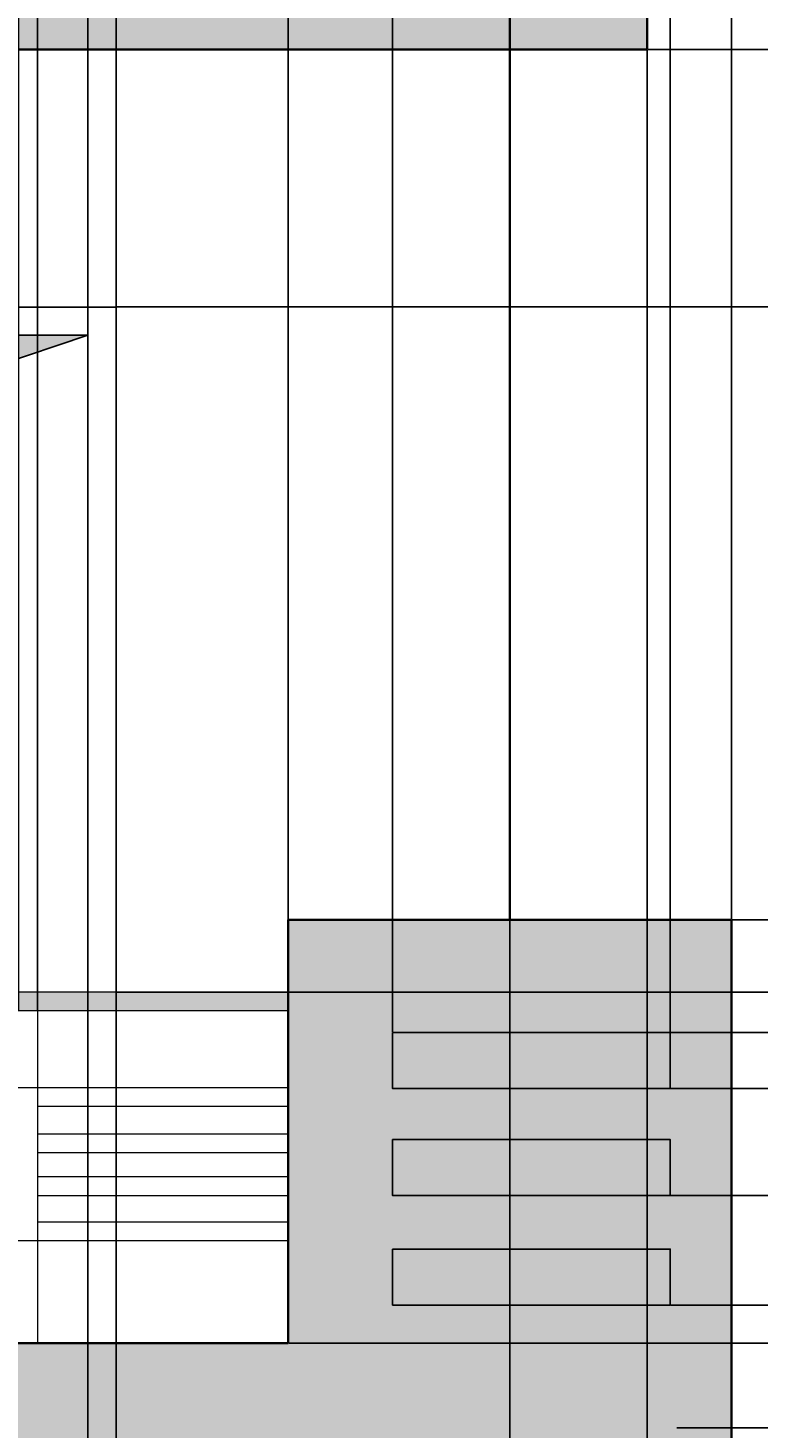
# Model space of a CAD drawing. Units: inches. Extents: x 62 to 566, y 66 to 528.
# Tile 17 of 20: x 365 to 443, y 298 to 447. Entities that reach past the tile are written whole.
import ezdxf

# ---------------------------------------------------------------- set-up
doc = ezdxf.new("R2010")
doc.units = ezdxf.units.IN
doc.header["$MEASUREMENT"] = 0
for name, color, linetype, lineweight in [('A-ANNO-DIMS', 2, 'Continuous', 18), ('A-DOOR', 4, 'Continuous', 25), ('A-ELEV', 7, 'Continuous', 35), ('A-FLOR-HRAL', 6, 'Continuous', 18), ('A-GLAZ', 3, 'Continuous', 25), ('A-WALL-PATT', 8, 'Continuous', 13)]:
    doc.layers.add(name, color=color, linetype=linetype, lineweight=lineweight)
doc.styles.get("Standard").update_dxf_attribs({"font": 'arial.ttf'})
doc.dimstyles.get("Standard").update_dxf_attribs({"dimtxt": 0.75, "dimasz": 0.18, "dimexe": 0.18, "dimexo": 0.0625, "dimgap": 0.09, "dimtad": 0, "dimtih": 1, "dimtoh": 1, "dimdec": 4, "dimzin": 0, "dimdsep": 46, "dimlunit": 4, "dimtxsty": 'Standard', "dimcen": 0.09, "dimadec": 0, "dimazin": 0, "dimtfac": 1, "dimtdec": 4, "dimtofl": 0, "dimtmove": 0, "dimatfit": 3, "dimfxl": 1, "dimtolj": 1, "dimtzin": 0, "dimarcsym": 0})

# ---------------------------------------------------------------- blocks, each defined once
blk = doc.blocks.new('*D23')
at = {"layer": 'A-ANNO-DIMS', "color": 0, "lineweight": -2, "transparency": 16777216}
for p, q in [((374.2, 344.78), (564.47, 344.78)), ((564.29, 344.6), (564.29, 308.57)), ((564.29, 271.59), (564.29, 307.62)), ((540.1, 271.41), (564.47, 271.41))]:
    blk.add_line(p, q, dxfattribs=at)
at = {"layer": 'A-ANNO-DIMS', "color": 0, "transparency": 16777216}
for points in [[(564.26, 344.6), (564.32, 344.6), (564.29, 344.78)], [(564.26, 271.59), (564.32, 271.59), (564.29, 271.41)]]:
    blk.add_solid(points, dxfattribs=at)
at = {"layer": 'Defpoints', "color": 0, "transparency": 16777216}
for p in [(374.14, 344.78), (564.29, 344.78), (540.04, 271.41)]:
    blk.add_point(p, dxfattribs=at)
at = {"layer": 'A-ANNO-DIMS', "color": 0, "transparency": 16777216, "insert": (564.29, 308.1), "char_height": 0.75, "attachment_point": 5}
blk.add_mtext('\\A1;73.37', dxfattribs=at)
blk = doc.blocks.new('*D24')
at = {"layer": 'A-ANNO-DIMS', "color": 0, "lineweight": -2, "transparency": 16777216}
for p, q in [((374.2, 417.71), (564.47, 417.71)), ((564.29, 417.53), (564.29, 381.72)), ((564.29, 344.96), (564.29, 380.77)), ((374.2, 344.78), (564.47, 344.78))]:
    blk.add_line(p, q, dxfattribs=at)
at = {"layer": 'A-ANNO-DIMS', "color": 0, "transparency": 16777216}
for points in [[(564.26, 417.53), (564.32, 417.53), (564.29, 417.71)], [(564.26, 344.96), (564.32, 344.96), (564.29, 344.78)]]:
    blk.add_solid(points, dxfattribs=at)
at = {"layer": 'Defpoints', "color": 0, "transparency": 16777216}
for p in [(374.14, 417.71), (564.29, 417.71), (374.14, 344.78)]:
    blk.add_point(p, dxfattribs=at)
at = {"layer": 'A-ANNO-DIMS', "color": 0, "transparency": 16777216, "insert": (564.29, 381.24), "char_height": 0.75, "attachment_point": 5}
blk.add_mtext('\\A1;72.92', dxfattribs=at)
blk = doc.blocks.new('*D41')
at = {"layer": 'A-ANNO-DIMS', "color": 0, "lineweight": -2, "transparency": 16777216}
for p, q in [((316.21, 417.64), (316.21, 65.94)), ((374.14, 417.64), (374.14, 65.94)), ((316.39, 66.12), (343.82, 66.12)), ((373.96, 66.12), (346.53, 66.12))]:
    blk.add_line(p, q, dxfattribs=at)
at = {"layer": 'A-ANNO-DIMS', "color": 0, "transparency": 16777216}
for points in [[(316.39, 66.15), (316.39, 66.09), (316.21, 66.12)], [(373.96, 66.15), (373.96, 66.09), (374.14, 66.12)]]:
    blk.add_solid(points, dxfattribs=at)
at = {"layer": 'Defpoints', "color": 0, "transparency": 16777216}
for p in [(316.21, 417.71), (374.14, 417.71), (374.14, 66.12)]:
    blk.add_point(p, dxfattribs=at)
at = {"layer": 'A-ANNO-DIMS', "color": 0, "transparency": 16777216, "insert": (345.17, 66.12), "char_height": 0.75, "attachment_point": 5}
blk.add_mtext('\\A1;57.93', dxfattribs=at)
blk = doc.blocks.new('*D42')
at = {"layer": 'A-ANNO-DIMS', "color": 0, "lineweight": -2, "transparency": 16777216}
for p, q in [((416.08, 445.04), (416.08, 65.94)), ((374.14, 417.64), (374.14, 65.94)), ((374.32, 66.12), (393.74, 66.12)), ((415.9, 66.12), (396.48, 66.12))]:
    blk.add_line(p, q, dxfattribs=at)
at = {"layer": 'A-ANNO-DIMS', "color": 0, "transparency": 16777216}
for points in [[(374.32, 66.15), (374.32, 66.09), (374.14, 66.12)], [(415.9, 66.15), (415.9, 66.09), (416.08, 66.12)]]:
    blk.add_solid(points, dxfattribs=at)
at = {"layer": 'Defpoints', "color": 0, "transparency": 16777216}
for p in [(416.08, 445.11), (374.14, 417.71), (416.08, 66.12)]:
    blk.add_point(p, dxfattribs=at)
at = {"layer": 'A-ANNO-DIMS', "color": 0, "transparency": 16777216, "insert": (395.11, 66.12), "char_height": 0.75, "attachment_point": 5}
blk.add_mtext('\\A1;41.95', dxfattribs=at)
blk = doc.blocks.new('*D43')
at = {"layer": 'A-ANNO-DIMS', "color": 0, "lineweight": -2, "transparency": 16777216}
for p, q in [((416.08, 445.04), (416.08, 65.94)), ((430.69, 445.04), (430.69, 65.94)), ((416.26, 66.12), (422.14, 66.12)), ((430.51, 66.12), (424.64, 66.12))]:
    blk.add_line(p, q, dxfattribs=at)
at = {"layer": 'A-ANNO-DIMS', "color": 0, "transparency": 16777216}
for points in [[(416.26, 66.15), (416.26, 66.09), (416.08, 66.12)], [(430.51, 66.15), (430.51, 66.09), (430.69, 66.12)]]:
    blk.add_solid(points, dxfattribs=at)
at = {"layer": 'Defpoints', "color": 0, "transparency": 16777216}
for p in [(416.08, 445.11), (430.69, 445.11), (430.69, 66.12)]:
    blk.add_point(p, dxfattribs=at)
at = {"layer": 'A-ANNO-DIMS', "color": 0, "transparency": 16777216, "insert": (423.39, 66.12), "char_height": 0.75, "attachment_point": 5}
blk.add_mtext('\\A1;14.61', dxfattribs=at)
blk = doc.blocks.new('*D52')
at = {"layer": 'A-ANNO-DIMS', "color": 0, "lineweight": -2, "transparency": 16777216}
for p, q in [((430.76, 445.11), (564.47, 445.11)), ((564.29, 444.93), (564.29, 431.87)), ((564.29, 417.89), (564.29, 430.94)), ((374.2, 417.71), (564.47, 417.71))]:
    blk.add_line(p, q, dxfattribs=at)
at = {"layer": 'A-ANNO-DIMS', "color": 0, "transparency": 16777216}
for points in [[(564.26, 444.93), (564.32, 444.93), (564.29, 445.11)], [(564.26, 417.89), (564.32, 417.89), (564.29, 417.71)]]:
    blk.add_solid(points, dxfattribs=at)
at = {"layer": 'Defpoints', "color": 0, "transparency": 16777216}
for p in [(430.69, 445.11), (564.29, 445.11), (374.14, 417.71)]:
    blk.add_point(p, dxfattribs=at)
at = {"layer": 'A-ANNO-DIMS', "color": 0, "transparency": 16777216, "insert": (564.29, 431.41), "char_height": 0.75, "attachment_point": 5}
blk.add_mtext('\\A1;27.4', dxfattribs=at)
blk = doc.blocks.new('*D53')
at = {"layer": 'A-ANNO-DIMS', "color": 0, "lineweight": -2, "transparency": 16777216}
for p, q in [((430.76, 462.04), (564.47, 462.04)), ((564.29, 461.86), (564.29, 454.05)), ((564.29, 445.29), (564.29, 453.1)), ((430.76, 445.11), (564.47, 445.11))]:
    blk.add_line(p, q, dxfattribs=at)
at = {"layer": 'A-ANNO-DIMS', "color": 0, "transparency": 16777216}
for points in [[(564.26, 461.86), (564.32, 461.86), (564.29, 462.04)], [(564.26, 445.29), (564.32, 445.29), (564.29, 445.11)]]:
    blk.add_solid(points, dxfattribs=at)
at = {"layer": 'Defpoints', "color": 0, "transparency": 16777216}
for p in [(430.69, 462.04), (564.29, 462.04), (430.69, 445.11)]:
    blk.add_point(p, dxfattribs=at)
at = {"layer": 'A-ANNO-DIMS', "color": 0, "transparency": 16777216, "insert": (564.29, 453.57), "char_height": 0.75, "attachment_point": 5}
blk.add_mtext('\\A1;16.936', dxfattribs=at)
blk = doc.blocks.new('*D63')
at = {"layer": 'A-ANNO-DIMS', "color": 0, "lineweight": -2, "transparency": 16777216}
for p, q in [((329.67, 219.79), (329.67, 527.47)), ((371.14, 233.72), (371.14, 527.47)), ((329.85, 527.29), (349.03, 527.29)), ((370.96, 527.29), (351.77, 527.29))]:
    blk.add_line(p, q, dxfattribs=at)
at = {"layer": 'A-ANNO-DIMS', "color": 0, "transparency": 16777216}
for points in [[(329.85, 527.32), (329.85, 527.26), (329.67, 527.29)], [(370.96, 527.32), (370.96, 527.26), (371.14, 527.29)]]:
    blk.add_solid(points, dxfattribs=at)
at = {"layer": 'Defpoints', "color": 0, "transparency": 16777216}
for p in [(371.14, 527.29), (371.14, 233.66), (329.67, 219.73)]:
    blk.add_point(p, dxfattribs=at)
at = {"layer": 'A-ANNO-DIMS', "color": 0, "transparency": 16777216, "insert": (350.4, 527.29), "char_height": 0.75, "attachment_point": 5}
blk.add_mtext('\\A1;41.47', dxfattribs=at)
blk = doc.blocks.new('*D64')
at = {"layer": 'A-ANNO-DIMS', "color": 0, "lineweight": -2, "transparency": 16777216}
for p, q in [((371.14, 233.72), (371.14, 527.47)), ((374.14, 236.72), (374.14, 527.47)), ((371.32, 527.29), (372.3, 527.29)), ((373.96, 527.29), (372.97, 527.29))]:
    blk.add_line(p, q, dxfattribs=at)
at = {"layer": 'A-ANNO-DIMS', "color": 0, "transparency": 16777216}
for points in [[(371.32, 527.32), (371.32, 527.26), (371.14, 527.29)], [(373.96, 527.32), (373.96, 527.26), (374.14, 527.29)]]:
    blk.add_solid(points, dxfattribs=at)
at = {"layer": 'Defpoints', "color": 0, "transparency": 16777216}
for p in [(374.14, 527.29), (374.14, 236.66), (371.14, 233.66)]:
    blk.add_point(p, dxfattribs=at)
at = {"layer": 'A-ANNO-DIMS', "color": 0, "transparency": 16777216, "insert": (372.64, 527.29), "char_height": 0.75, "attachment_point": 5}
blk.add_mtext('\\A1;3', dxfattribs=at)
blk = doc.blocks.new('*D77')
at = {"layer": 'A-ANNO-DIMS', "color": 0, "lineweight": -2, "transparency": 16777216}
for p, q in [((363.76, 342.84), (363.76, 527.47)), ((365.76, 342.84), (365.76, 527.47)), ((363.94, 527.29), (364.43, 527.29)), ((365.58, 527.29), (365.1, 527.29))]:
    blk.add_line(p, q, dxfattribs=at)
at = {"layer": 'A-ANNO-DIMS', "color": 0, "transparency": 16777216}
for points in [[(363.94, 527.32), (363.94, 527.26), (363.76, 527.29)], [(365.58, 527.32), (365.58, 527.26), (365.76, 527.29)]]:
    blk.add_solid(points, dxfattribs=at)
at = {"layer": 'Defpoints', "color": 0, "transparency": 16777216}
for p in [(365.76, 527.29), (363.76, 342.78), (365.76, 342.78)]:
    blk.add_point(p, dxfattribs=at)
at = {"layer": 'A-ANNO-DIMS', "color": 0, "transparency": 16777216, "insert": (364.76, 527.29), "char_height": 0.75, "attachment_point": 5}
blk.add_mtext('\\A1;2', dxfattribs=at)
blk = doc.blocks.new('*D78')
at = {"layer": 'A-ANNO-DIMS', "color": 0, "lineweight": -2, "transparency": 16777216}
for p, q in [((365.76, 342.84), (365.76, 527.47)), ((392.48, 342.84), (392.48, 527.47)), ((365.94, 527.29), (377.47, 527.29)), ((392.3, 527.29), (380.78, 527.29))]:
    blk.add_line(p, q, dxfattribs=at)
at = {"layer": 'A-ANNO-DIMS', "color": 0, "transparency": 16777216}
for points in [[(365.94, 527.32), (365.94, 527.26), (365.76, 527.29)], [(392.3, 527.32), (392.3, 527.26), (392.48, 527.29)]]:
    blk.add_solid(points, dxfattribs=at)
at = {"layer": 'Defpoints', "color": 0, "transparency": 16777216}
for p in [(392.48, 527.29), (365.76, 342.78), (392.48, 342.78)]:
    blk.add_point(p, dxfattribs=at)
at = {"layer": 'A-ANNO-DIMS', "color": 0, "transparency": 16777216, "insert": (379.12, 527.29), "char_height": 0.75, "attachment_point": 5}
blk.add_mtext('\\A1;26.715', dxfattribs=at)
blk = doc.blocks.new('*D79')
at = {"layer": 'A-ANNO-DIMS', "color": 0, "lineweight": -2, "transparency": 16777216}
for p, q in [((392.48, 352.55), (392.48, 527.47)), ((403.58, 340.55), (403.58, 527.47)), ((392.66, 527.29), (396.42, 527.29)), ((403.4, 527.29), (399.64, 527.29))]:
    blk.add_line(p, q, dxfattribs=at)
at = {"layer": 'A-ANNO-DIMS', "color": 0, "transparency": 16777216}
for points in [[(392.66, 527.32), (392.66, 527.26), (392.48, 527.29)], [(403.4, 527.32), (403.4, 527.26), (403.58, 527.29)]]:
    blk.add_solid(points, dxfattribs=at)
at = {"layer": 'Defpoints', "color": 0, "transparency": 16777216}
for p in [(403.58, 527.29), (392.48, 352.48), (403.58, 340.49)]:
    blk.add_point(p, dxfattribs=at)
at = {"layer": 'A-ANNO-DIMS', "color": 0, "transparency": 16777216, "insert": (398.03, 527.29), "char_height": 0.75, "attachment_point": 5}
blk.add_mtext('\\A1;11.106', dxfattribs=at)
blk = doc.blocks.new('*D80')
at = {"layer": 'A-ANNO-DIMS', "color": 0, "lineweight": -2, "transparency": 16777216}
for p, q in [((403.58, 340.55), (403.58, 527.47)), ((433.16, 340.55), (433.16, 527.47)), ((403.76, 527.29), (417.01, 527.29)), ((432.98, 527.29), (419.74, 527.29))]:
    blk.add_line(p, q, dxfattribs=at)
at = {"layer": 'A-ANNO-DIMS', "color": 0, "transparency": 16777216}
for points in [[(403.76, 527.32), (403.76, 527.26), (403.58, 527.29)], [(432.98, 527.32), (432.98, 527.26), (433.16, 527.29)]]:
    blk.add_solid(points, dxfattribs=at)
at = {"layer": 'Defpoints', "color": 0, "transparency": 16777216}
for p in [(433.16, 527.29), (403.58, 340.49), (433.16, 340.49)]:
    blk.add_point(p, dxfattribs=at)
at = {"layer": 'A-ANNO-DIMS', "color": 0, "transparency": 16777216, "insert": (418.37, 527.29), "char_height": 0.75, "attachment_point": 5}
blk.add_mtext('\\A1;29.58', dxfattribs=at)
blk = doc.blocks.new('*D81')
at = {"layer": 'A-ANNO-DIMS', "color": 0, "lineweight": -2, "transparency": 16777216}
for p, q in [((433.16, 340.55), (433.16, 527.47)), ((439.69, 352.55), (439.69, 527.47)), ((433.34, 527.29), (435.07, 527.29)), ((439.51, 527.29), (437.78, 527.29))]:
    blk.add_line(p, q, dxfattribs=at)
at = {"layer": 'A-ANNO-DIMS', "color": 0, "transparency": 16777216}
for points in [[(433.34, 527.32), (433.34, 527.26), (433.16, 527.29)], [(439.51, 527.32), (439.51, 527.26), (439.69, 527.29)]]:
    blk.add_solid(points, dxfattribs=at)
at = {"layer": 'Defpoints', "color": 0, "transparency": 16777216}
for p in [(439.69, 527.29), (439.69, 352.48), (433.16, 340.49)]:
    blk.add_point(p, dxfattribs=at)
at = {"layer": 'A-ANNO-DIMS', "color": 0, "transparency": 16777216, "insert": (436.43, 527.29), "char_height": 0.75, "attachment_point": 5}
blk.add_mtext('\\A1;6.524', dxfattribs=at)
blk = doc.blocks.new('*D91')
at = {"layer": 'A-ANNO-DIMS', "color": 0, "lineweight": -2, "transparency": 16777216}
for p, q in [((433.87, 298.4), (564.47, 298.4)), ((564.29, 298.22), (564.29, 297.15)), ((564.29, 295.13), (564.29, 296.2)), ((433.87, 294.95), (564.47, 294.95))]:
    blk.add_line(p, q, dxfattribs=at)
at = {"layer": 'A-ANNO-DIMS', "color": 0, "transparency": 16777216}
for points in [[(564.26, 298.22), (564.32, 298.22), (564.29, 298.4)], [(564.26, 295.13), (564.32, 295.13), (564.29, 294.95)]]:
    blk.add_solid(points, dxfattribs=at)
at = {"layer": 'Defpoints', "color": 0, "transparency": 16777216}
for p in [(433.81, 298.4), (564.29, 298.4), (433.81, 294.95)]:
    blk.add_point(p, dxfattribs=at)
at = {"layer": 'A-ANNO-DIMS', "color": 0, "transparency": 16777216, "insert": (564.29, 296.67), "char_height": 0.75, "attachment_point": 5}
blk.add_mtext('\\A1;3.449', dxfattribs=at)
blk = doc.blocks.new('*D92')
at = {"layer": 'A-ANNO-DIMS', "color": 0, "lineweight": -2, "transparency": 16777216}
for p, q in [((392.54, 307.41), (564.47, 307.41)), ((564.29, 307.23), (564.29, 303.38)), ((564.29, 298.58), (564.29, 302.43)), ((433.87, 298.4), (564.47, 298.4))]:
    blk.add_line(p, q, dxfattribs=at)
at = {"layer": 'A-ANNO-DIMS', "color": 0, "transparency": 16777216}
for points in [[(564.26, 307.23), (564.32, 307.23), (564.29, 307.41)], [(564.26, 298.58), (564.32, 298.58), (564.29, 298.4)]]:
    blk.add_solid(points, dxfattribs=at)
at = {"layer": 'Defpoints', "color": 0, "transparency": 16777216}
for p in [(392.48, 307.41), (564.29, 307.41), (433.81, 298.4)]:
    blk.add_point(p, dxfattribs=at)
at = {"layer": 'A-ANNO-DIMS', "color": 0, "transparency": 16777216, "insert": (564.29, 302.91), "char_height": 0.75, "attachment_point": 5}
blk.add_mtext('\\A1;9.014', dxfattribs=at)
blk = doc.blocks.new('*D93')
at = {"layer": 'A-ANNO-DIMS', "color": 0, "lineweight": -2, "transparency": 16777216}
for p, q in [((433.23, 311.47), (564.47, 311.47)), ((564.29, 311.29), (564.29, 309.92)), ((564.29, 307.59), (564.29, 308.97)), ((392.54, 307.41), (564.47, 307.41))]:
    blk.add_line(p, q, dxfattribs=at)
at = {"layer": 'A-ANNO-DIMS', "color": 0, "transparency": 16777216}
for points in [[(564.26, 311.29), (564.32, 311.29), (564.29, 311.47)], [(564.26, 307.59), (564.32, 307.59), (564.29, 307.41)]]:
    blk.add_solid(points, dxfattribs=at)
at = {"layer": 'Defpoints', "color": 0, "transparency": 16777216}
for p in [(433.16, 311.47), (564.29, 311.47), (392.48, 307.41)]:
    blk.add_point(p, dxfattribs=at)
at = {"layer": 'A-ANNO-DIMS', "color": 0, "transparency": 16777216, "insert": (564.29, 309.44), "char_height": 0.75, "attachment_point": 5}
blk.add_mtext('\\A1;4.061', dxfattribs=at)
blk = doc.blocks.new('*D94')
at = {"layer": 'A-ANNO-DIMS', "color": 0, "lineweight": -2, "transparency": 16777216}
for p, q in [((433.23, 323.13), (564.47, 323.13)), ((564.29, 322.95), (564.29, 317.78)), ((564.29, 311.65), (564.29, 316.83)), ((433.23, 311.47), (564.47, 311.47))]:
    blk.add_line(p, q, dxfattribs=at)
at = {"layer": 'A-ANNO-DIMS', "color": 0, "transparency": 16777216}
for points in [[(564.26, 322.95), (564.32, 322.95), (564.29, 323.13)], [(564.26, 311.65), (564.32, 311.65), (564.29, 311.47)]]:
    blk.add_solid(points, dxfattribs=at)
at = {"layer": 'Defpoints', "color": 0, "transparency": 16777216}
for p in [(433.16, 323.13), (564.29, 323.13), (433.16, 311.47)]:
    blk.add_point(p, dxfattribs=at)
at = {"layer": 'A-ANNO-DIMS', "color": 0, "transparency": 16777216, "insert": (564.29, 317.3), "char_height": 0.75, "attachment_point": 5}
blk.add_mtext('\\A1;11.66', dxfattribs=at)
blk = doc.blocks.new('*D95')
at = {"layer": 'A-ANNO-DIMS', "color": 0, "lineweight": -2, "transparency": 16777216}
for p, q in [((433.23, 334.52), (564.47, 334.52)), ((564.29, 334.34), (564.29, 329.3)), ((564.29, 323.31), (564.29, 328.35)), ((433.23, 323.13), (564.47, 323.13))]:
    blk.add_line(p, q, dxfattribs=at)
at = {"layer": 'A-ANNO-DIMS', "color": 0, "transparency": 16777216}
for points in [[(564.26, 334.34), (564.32, 334.34), (564.29, 334.52)], [(564.26, 323.31), (564.32, 323.31), (564.29, 323.13)]]:
    blk.add_solid(points, dxfattribs=at)
at = {"layer": 'Defpoints', "color": 0, "transparency": 16777216}
for p in [(433.16, 334.52), (564.29, 334.52), (433.16, 323.13)]:
    blk.add_point(p, dxfattribs=at)
at = {"layer": 'A-ANNO-DIMS', "color": 0, "transparency": 16777216, "insert": (564.29, 328.83), "char_height": 0.75, "attachment_point": 5}
blk.add_mtext('\\A1;11.388', dxfattribs=at)
blk = doc.blocks.new('*D96')
at = {"layer": 'A-ANNO-DIMS', "color": 0, "lineweight": -2, "transparency": 16777216}
for p, q in [((433.23, 340.49), (564.47, 340.49)), ((564.29, 340.31), (564.29, 337.98)), ((564.29, 334.7), (564.29, 337.03)), ((433.23, 334.52), (564.47, 334.52))]:
    blk.add_line(p, q, dxfattribs=at)
at = {"layer": 'A-ANNO-DIMS', "color": 0, "transparency": 16777216}
for points in [[(564.26, 340.31), (564.32, 340.31), (564.29, 340.49)], [(564.26, 334.7), (564.32, 334.7), (564.29, 334.52)]]:
    blk.add_solid(points, dxfattribs=at)
at = {"layer": 'Defpoints', "color": 0, "transparency": 16777216}
for p in [(433.16, 340.49), (564.29, 340.49), (433.16, 334.52)]:
    blk.add_point(p, dxfattribs=at)
at = {"layer": 'A-ANNO-DIMS', "color": 0, "transparency": 16777216, "insert": (564.29, 337.5), "char_height": 0.75, "attachment_point": 5}
blk.add_mtext('\\A1;5.965', dxfattribs=at)
blk = doc.blocks.new('*D97')
at = {"layer": 'A-ANNO-DIMS', "color": 0, "lineweight": -2, "transparency": 16777216}
for p, q in [((439.75, 352.48), (564.47, 352.48)), ((564.29, 352.3), (564.29, 346.96)), ((564.29, 340.67), (564.29, 346.01)), ((433.23, 340.49), (564.47, 340.49))]:
    blk.add_line(p, q, dxfattribs=at)
at = {"layer": 'A-ANNO-DIMS', "color": 0, "transparency": 16777216}
for points in [[(564.26, 352.3), (564.32, 352.3), (564.29, 352.48)], [(564.26, 340.67), (564.32, 340.67), (564.29, 340.49)]]:
    blk.add_solid(points, dxfattribs=at)
at = {"layer": 'Defpoints', "color": 0, "transparency": 16777216}
for p in [(439.69, 352.48), (564.29, 352.48), (433.16, 340.49)]:
    blk.add_point(p, dxfattribs=at)
at = {"layer": 'A-ANNO-DIMS', "color": 0, "transparency": 16777216, "insert": (564.29, 346.49), "char_height": 0.75, "attachment_point": 5}
blk.add_mtext('\\A1;11.998', dxfattribs=at)

msp = doc.modelspace()

# ---------------------------------------------------------------- hatches: boundary and pattern name
at = {"layer": 'A-WALL-PATT'}
h = msp.add_hatch(color=256, dxfattribs=at)
h.dxf.hatch_style = 1
h.paths.add_polyline_path([(416.0836, 462.0423), (125.9418, 462.0423), (125.9418, 414.3686), (125.9418, 270.3686), (125.9418, 126.3686), (142.3851, 126.3686), (142.3851, 270.3686), (142.3851, 414.3686), (142.3851, 445.1064), (284.2021, 445.1064), (416.0836, 445.1064)])
h.paths.add_polyline_path([(435.3945, 503.0423), (426.3652, 503.0423), (120.4058, 503.0423), (120.4058, 501.0423), (125.9418, 501.0423), (416.0836, 501.0423), (426.3652, 501.0423), (430.6938, 501.0423), (435.3945, 501.0423)])
h.paths.add_polyline_path([(439.6878, 352.4848), (392.4793, 352.4848), (392.4793, 307.4128), (217.2752, 307.4128), (217.2752, 295.4098), (217.2752, 271.4128), (272.0586, 271.4128), (439.6878, 271.4128)])
h.paths.add_polyline_path([(248.0143, 297.1682), (255.6783, 297.1682), (255.6783, 280.0423), (248.0143, 280.0423)], flags=16)
h.paths.add_polyline_path([(235.4641, 280.0423), (227.8001, 280.0423), (227.8001, 297.1682), (235.4641, 297.1682)], flags=16)
h.paths.add_polyline_path([(270.4427, 297.1682), (278.1067, 297.1682), (278.1067, 280.0423), (270.4427, 280.0423)], flags=16)
h.paths.add_polyline_path([(296.3755, 297.1682), (304.0395, 297.1682), (304.0395, 280.0423), (296.3755, 280.0423)], flags=16)
h.paths.add_polyline_path([(319.2543, 297.1682), (326.9183, 297.1682), (326.9183, 280.0423), (319.2543, 280.0423)], flags=16)
h.paths.add_polyline_path([(341.2622, 297.1682), (348.9262, 297.1682), (348.9262, 280.0423), (341.2622, 280.0423)], flags=16)
h.paths.add_polyline_path([(389.2857, 298.3985), (433.8102, 298.3985), (433.8102, 294.9497), (389.2857, 294.9497)], flags=16)
h.paths.add_polyline_path([(389.2857, 291.6038), (433.8102, 291.6038), (433.8102, 288.155), (389.2857, 288.155)], flags=16)
h.paths.add_polyline_path([(389.2857, 284.9607), (433.8102, 284.9607), (433.8102, 281.5119), (389.2857, 281.5119)], flags=16)
h.paths.add_polyline_path([(403.5849, 311.4736), (403.5849, 317.4388), (433.1636, 317.4388), (433.1636, 311.4736)], flags=16)
h.paths.add_polyline_path([(403.5849, 323.1329), (403.5849, 329.0982), (433.1636, 329.0982), (433.1636, 323.1329)], flags=16)
h.paths.add_polyline_path([(403.5849, 334.5211), (403.5849, 340.4863), (433.1636, 340.4863), (433.1636, 334.5211)], flags=16)
h.paths.add_polyline_path([(272.0586, 160.3545), (217.2752, 160.3545), (217.2752, 129.0504), (217.2752, 126.3686), (272.0586, 126.3686)], flags=17)
h.paths.add_polyline_path([(220.5897, 149.5749), (220.5897, 152.296), (267.7931, 152.296), (267.7931, 149.5749)], flags=16)
h.paths.add_polyline_path([(267.7931, 146.6724), (267.7931, 143.9513), (220.5897, 143.9513), (220.5897, 146.6724)], flags=16)
h.paths.add_polyline_path([(220.5897, 155.3799), (220.5897, 158.101), (267.7931, 158.101), (267.7931, 155.3799)], flags=16)
h.paths.add_polyline_path([(267.7931, 140.686), (267.7931, 137.9649), (220.5897, 137.9649), (220.5897, 140.686)], flags=16)
h.paths.add_polyline_path([(267.7931, 135.516), (267.7931, 132.7949), (220.5897, 132.7949), (220.5897, 135.516)], flags=16)
h = msp.add_hatch(color=256, dxfattribs=at)
h.dxf.hatch_style = 1
h.paths.add_polyline_path([(416.0836, 501.0423), (282.3509, 501.0423), (282.3509, 465.0423), (416.0836, 465.0423)])
h.paths.add_polyline_path([(284.2021, 420.597), (272.0586, 420.597), (272.0586, 309.5388), (272.0586, 307.4128), (284.2021, 307.4128)], flags=17)
h.paths.add_polyline_path([(284.2021, 445.1064), (142.3851, 445.1064), (142.3851, 414.3686), (142.3851, 270.3686), (142.3851, 126.3686), (163.6548, 126.3686), (163.6548, 270.5016), (163.6548, 414.5016), (163.6548, 427.4752), (284.2021, 427.4752)])
h.paths.add_polyline_path([(235.4641, 297.1682), (227.8001, 297.1682), (227.8001, 280.0423), (235.4641, 280.0423)], flags=17)
h.paths.add_polyline_path([(255.6783, 297.1682), (248.0143, 297.1682), (248.0143, 280.0423), (255.6783, 280.0423)], flags=17)
h.paths.add_polyline_path([(278.1067, 297.1682), (270.4427, 297.1682), (270.4427, 280.0423), (278.1067, 280.0423)], flags=17)
h.paths.add_polyline_path([(304.0395, 297.1682), (296.3755, 297.1682), (296.3755, 280.0423), (304.0395, 280.0423)])
h.paths.add_polyline_path([(326.9183, 297.1682), (319.2543, 297.1682), (319.2543, 280.0423), (326.9183, 280.0423)])
h.paths.add_polyline_path([(348.9262, 297.1682), (341.2622, 297.1682), (341.2622, 280.0423), (348.9262, 280.0423)])
h.paths.add_polyline_path([(433.8102, 284.9607), (389.2857, 284.9607), (389.2857, 281.5119), (433.8102, 281.5119)])
h.paths.add_polyline_path([(433.8102, 291.6038), (389.2857, 291.6038), (389.2857, 288.155), (433.8102, 288.155)])
h.paths.add_polyline_path([(433.8102, 298.3985), (389.2857, 298.3985), (389.2857, 294.9497), (433.8102, 294.9497)])
h.paths.add_polyline_path([(433.1636, 317.4388), (403.5849, 317.4388), (403.5849, 311.4736), (433.1636, 311.4736)])
h.paths.add_polyline_path([(433.1636, 329.0982), (403.5849, 329.0982), (403.5849, 323.1329), (433.1636, 323.1329)])
h.paths.add_polyline_path([(433.1636, 340.4863), (403.5849, 340.4863), (403.5849, 334.5211), (433.1636, 334.5211)])
h.paths.add_polyline_path([(284.2021, 271.4128), (272.0586, 271.4128), (272.0586, 160.3545), (272.0586, 126.3686), (284.2021, 126.3686)])
h.paths.add_polyline_path([(267.7931, 158.101), (220.5897, 158.101), (220.5897, 155.3799), (267.7931, 155.3799)], flags=17)
h.paths.add_polyline_path([(267.7931, 152.296), (220.5897, 152.296), (220.5897, 149.5749), (267.7931, 149.5749)], flags=17)
h.paths.add_polyline_path([(267.7931, 146.6724), (220.5897, 146.6724), (220.5897, 143.9513), (267.7931, 143.9513)], flags=17)
h.paths.add_polyline_path([(267.7931, 140.686), (220.5897, 140.686), (220.5897, 137.9649), (267.7931, 137.9649)], flags=17)
h.paths.add_polyline_path([(267.7931, 135.516), (220.5897, 135.516), (220.5897, 132.7949), (267.7931, 132.7949)], flags=17)
h.paths.add_polyline_path([(148.2354, 493.4274), (140.5713, 493.4274), (140.5713, 476.3015), (148.2354, 476.3015)])
h.paths.add_polyline_path([(163.2545, 493.4274), (155.5905, 493.4274), (155.5905, 476.3015), (163.2545, 476.3015)])
h.paths.add_polyline_path([(177.9243, 493.7764), (170.2603, 493.7764), (170.2603, 476.6506), (177.9243, 476.6506)])
h.paths.add_polyline_path([(193.9913, 493.7764), (186.3273, 493.7764), (186.3273, 476.6506), (193.9913, 476.6506)])
h.paths.add_polyline_path([(209.709, 493.7764), (202.045, 493.7764), (202.045, 476.6506), (209.709, 476.6506)])
h = msp.add_hatch(color=256, dxfattribs=at)
h.dxf.hatch_style = 1
h.paths.add_polyline_path([(430.6938, 462.0423), (416.0836, 462.0423), (416.0836, 445.1064), (430.6938, 445.1064)])
h.paths.add_polyline_path([(169.0431, 420.597), (284.2021, 420.597), (284.2021, 426.4752), (164.6548, 426.4752), (164.6548, 414.5016), (164.6548, 126.3686), (169.0431, 126.3686)])
h = msp.add_hatch(color=256, dxfattribs=at)
h.dxf.hatch_style = 1
h.paths.add_polyline_path([(371.1373, 233.6618), (319.2101, 233.6618), (319.2101, 129.3686), (329.6665, 129.3686), (329.6665, 219.7304)])
h.paths.add_polyline_path([(371.1373, 414.7059), (319.2101, 414.7059), (319.2101, 344.7821), (329.6665, 344.7821), (329.6665, 400.7745)])
h.paths.add_polyline_path([(392.4793, 344.7821), (284.2021, 344.7821), (284.2021, 342.7821), (392.4793, 342.7821)])

# ---------------------------------------------------------------- linework, layer by layer
at = {"layer": 'A-DOOR'}
msp.add_line((371.1373, 414.7059), (329.6665, 400.7745), dxfattribs=at)
for points in [[(316.2101, 344.7821), (316.2101, 417.7059), (374.1373, 417.7059), (374.1373, 344.7821)], [(319.2101, 344.7821), (319.2101, 414.7059), (371.1373, 414.7059), (371.1373, 344.7821)], [(374.1373, 307.4128), (316.2101, 307.4128)]]:
    msp.add_lwpolyline(points, dxfattribs=at)
at = {"layer": 'A-ELEV'}
for p, q in [((416.0836, 352.4848), (416.0836, 462.0423)), ((430.6938, 445.1064), (430.6938, 462.0423)), ((284.2021, 445.1064), (416.0836, 445.1064)), ((416.0836, 445.1064), (430.6938, 445.1064)), ((392.4793, 307.4128), (392.4793, 352.4848)), ((392.4793, 352.4848), (439.6878, 352.4848)), ((439.6878, 352.4848), (439.6878, 271.4128)), ((217.2752, 307.4128), (392.4793, 307.4128))]:
    msp.add_line(p, q, dxfattribs=at)
at = {"layer": 'A-FLOR-HRAL'}
for p, q in [((392.4793, 344.7821), (284.2021, 344.7821)), ((392.4793, 342.7821), (284.2021, 342.7821)), ((365.764, 342.7821), (365.764, 307.4128)), ((392.4793, 334.6119), (284.2021, 334.6119)), ((392.4793, 332.6119), (365.764, 332.6119)), ((392.4793, 329.6741), (365.764, 329.6741)), ((392.4793, 327.6741), (365.764, 327.6741)), ((392.4793, 325.1162), (365.764, 325.1162)), ((392.4793, 323.1162), (365.764, 323.1162)), ((392.4793, 320.3051), (365.764, 320.3051)), ((392.4793, 318.3051), (284.2021, 318.3051))]:
    msp.add_line(p, q, dxfattribs=at)
at = {"layer": 'A-GLAZ'}
for points in [[(403.5849, 340.4863), (433.1636, 340.4863), (433.1636, 334.5211), (403.5849, 334.5211)], [(403.5849, 329.0982), (433.1636, 329.0982), (433.1636, 323.1329), (403.5849, 323.1329)], [(403.5849, 317.4388), (433.1636, 317.4388), (433.1636, 311.4736), (403.5849, 311.4736)]]:
    msp.add_lwpolyline(points, close=True, dxfattribs=at)

# ---------------------------------------------------------------- dimensions: what is measured, and where the dimension line sits
at = {"layer": 'A-ANNO-DIMS'}
for base, p1, p2, override, picture, middle in [((371.1373, 527.2923), (329.6665, 219.7304), (371.1373, 233.6618), {"dimdec": 2, "dimlfac": 1, "dimrnd": 0, "dimzin": 0, "dimdsep": 46, "dimlunit": 2}, '*D63', (350.4019, 527.2923)), ((365.764, 527.2923), (363.764, 342.7821), (365.764, 342.7821), {"dimdec": 0, "dimlfac": 1, "dimrnd": 0, "dimzin": 0, "dimdsep": 46, "dimlunit": 2}, '*D77', (364.764, 527.2923)), ((392.4793, 527.2923), (365.764, 342.7821), (392.4793, 342.7821), {"dimdec": 3, "dimlfac": 1, "dimrnd": 0, "dimzin": 0, "dimdsep": 46, "dimlunit": 2}, '*D78', (379.1216, 527.2923)), ((374.1373, 527.2923), (371.1373, 233.6618), (374.1373, 236.6618), {"dimdec": 0, "dimlfac": 1, "dimrnd": 0, "dimzin": 0, "dimdsep": 46, "dimlunit": 2}, '*D64', (372.6373, 527.2923)), ((403.5849, 527.2923), (392.4793, 352.4848), (403.5849, 340.4863), {"dimdec": 3, "dimlfac": 1, "dimrnd": 0, "dimzin": 0, "dimdsep": 46, "dimlunit": 2}, '*D79', (398.0321, 527.2923)), ((433.1636, 527.2923), (403.5849, 340.4863), (433.1636, 340.4863), {"dimdec": 2, "dimlfac": 1, "dimrnd": 0, "dimzin": 0, "dimdsep": 46, "dimlunit": 2}, '*D80', (418.3743, 527.2923)), ((439.6878, 527.2923), (433.1636, 340.4863), (439.6878, 352.4848), {"dimdec": 3, "dimlfac": 1, "dimrnd": 0, "dimzin": 0, "dimdsep": 46, "dimlunit": 2}, '*D81', (436.4257, 527.2923)), ((416.0836, 66.1186), (374.1373, 417.7059), (416.0836, 445.1064), {"dimdec": 2, "dimlfac": 1, "dimrnd": 0, "dimzin": 0, "dimdsep": 46, "dimlunit": 2}, '*D42', (395.1104, 66.1186)), ((430.6938, 66.1186), (416.0836, 445.1064), (430.6938, 445.1064), {"dimdec": 2, "dimlfac": 1, "dimrnd": 0, "dimzin": 0, "dimdsep": 46, "dimlunit": 2}, '*D43', (423.3887, 66.1186)), ((374.1373, 66.1186), (316.2101, 417.7059), (374.1373, 417.7059), {"dimdec": 2, "dimlfac": 1, "dimrnd": 0, "dimzin": 0, "dimdsep": 46, "dimlunit": 2}, '*D41', (345.1737, 66.1186))]:
    dim = msp.add_linear_dim(base=base, p1=p1, p2=p2, dimstyle='Standard', override=override, dxfattribs=at)
    dim.commit()
    dim.dimension.update_dxf_attribs({"geometry": picture, "text_midpoint": middle})
for base, p1, p2, override, picture, middle in [((564.2868, 462.0423), (430.6938, 445.1064), (430.6938, 462.0423), {"dimdec": 3, "dimlfac": 1, "dimrnd": 0, "dimzin": 0, "dimdsep": 46, "dimlunit": 2}, '*D53', (564.2868, 453.5744)), ((564.2868, 445.1064), (374.1373, 417.7059), (430.6938, 445.1064), {"dimdec": 1, "dimlfac": 1, "dimrnd": 0, "dimzin": 0, "dimdsep": 46, "dimlunit": 2}, '*D52', (564.2868, 431.4062)), ((564.2868, 417.7059), (374.1373, 344.7821), (374.1373, 417.7059), {"dimdec": 2, "dimlfac": 1, "dimrnd": 0, "dimzin": 0, "dimdsep": 46, "dimlunit": 2}, '*D24', (564.2868, 381.244)), ((564.28678, 352.4848), (433.16362, 340.48631), (439.68784, 352.4848), {"dimdec": 3, "dimlfac": 1, "dimrnd": 0, "dimzin": 0, "dimdsep": 46, "dimlunit": 2}, '*D97', (564.28678, 346.48556)), ((564.2868, 344.7821), (540.0368, 271.4128), (374.1373, 344.7821), {"dimdec": 2, "dimlfac": 1, "dimrnd": 0, "dimzin": 0, "dimdsep": 46, "dimlunit": 2}, '*D23', (564.2868, 308.0974)), ((564.2868, 340.4863), (433.1636, 334.5211), (433.1636, 340.4863), {"dimdec": 3, "dimlfac": 1, "dimrnd": 0, "dimzin": 0, "dimdsep": 46, "dimlunit": 2}, '*D96', (564.2868, 337.5037)), ((564.2868, 334.5211), (433.1636, 323.1329), (433.1636, 334.5211), {"dimdec": 3, "dimlfac": 1, "dimrnd": 0, "dimzin": 0, "dimdsep": 46, "dimlunit": 2}, '*D95', (564.2868, 328.827)), ((564.2868, 323.1329), (433.1636, 311.4736), (433.1636, 323.1329), {"dimdec": 2, "dimlfac": 1, "dimrnd": 0, "dimzin": 0, "dimdsep": 46, "dimlunit": 2}, '*D94', (564.2868, 317.3033)), ((564.2868, 311.4736), (392.4793, 307.4128), (433.1636, 311.4736), {"dimdec": 3, "dimlfac": 1, "dimrnd": 0, "dimzin": 0, "dimdsep": 46, "dimlunit": 2}, '*D93', (564.2868, 309.4432)), ((564.2868, 307.4128), (433.8102, 298.3985), (392.4793, 307.4128), {"dimdec": 3, "dimlfac": 1, "dimrnd": 0, "dimzin": 0, "dimdsep": 46, "dimlunit": 2}, '*D92', (564.2868, 302.9056)), ((564.2868, 298.3985), (433.8102, 294.9497), (433.8102, 298.3985), {"dimdec": 3, "dimlfac": 1, "dimrnd": 0, "dimzin": 0, "dimdsep": 46, "dimlunit": 2}, '*D91', (564.2868, 296.6741))]:
    dim = msp.add_linear_dim(base=base, p1=p1, p2=p2, angle=90, dimstyle='Standard', override=override, dxfattribs=at)
    dim.commit()
    dim.dimension.update_dxf_attribs({"geometry": picture, "text_midpoint": middle})

doc.saveas('drawing.dxf')
